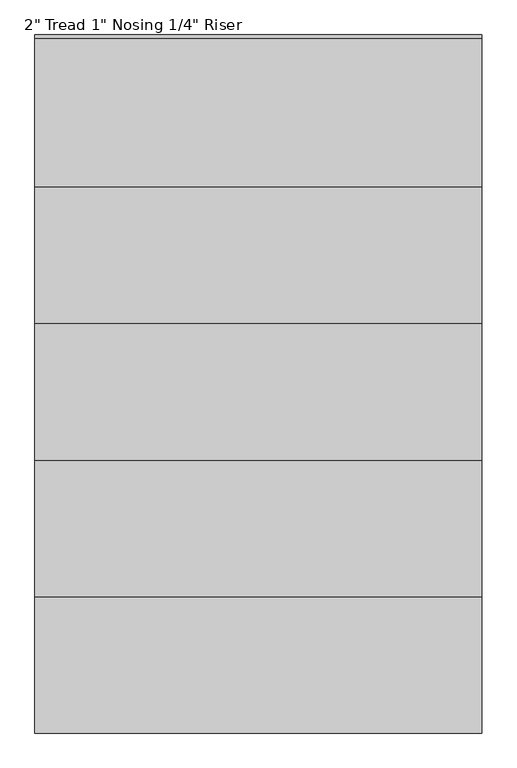
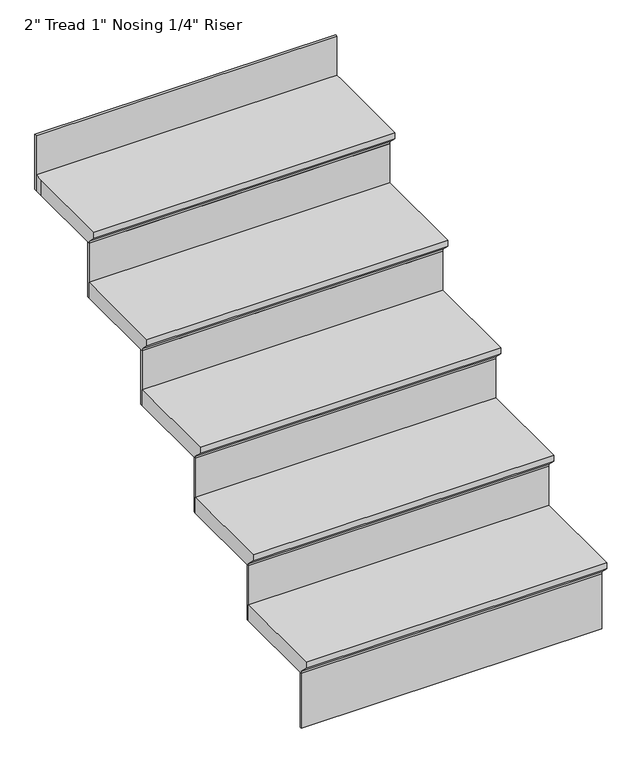
"""IFC4 building model written with IfcOpenShell, lengths in millimetres: stair flight geometry."""

from ifc_helpers import new_model, si_unit, origin, place, context, project, spatial, faceted_brep, source, transform, mapped, element, save


def stair_flight_150202ba(model_context):
    return source(origin(), model_context, "Body", "Brep", [
        faceted_brep([(9871.2423568, -9537.7746824, 1216.1921053), (9871.2423568, -9537.7746824, 1235.2421053), (8956.8423568, -9537.7746824, 1235.2421053), (8956.8423568, -9537.7746824, 1216.1921053), (9871.2423568, -9512.3746824, 1190.7921053), (8956.8423568, -9512.3746824, 1190.7921053), (9871.2423568, -9232.9746824, 1235.2421053), (8956.8423568, -9232.9746824, 1235.2421053), (8956.8423568, -9512.3746824, 1184.4421053), (8956.8423568, -9232.9746824, 1184.4421053), (9871.2423568, -9232.9746824, 1184.4421053), (9871.2423568, -9512.3746824, 1184.4421053)], [[[0, 1, 2, 3]], [[4, 0, 3, 5]], [[2, 1, 6, 7]], [[8, 9, 10, 11]], [[2, 7, 9, 8, 5, 3]], [[8, 11, 4, 5]], [[6, 1, 0, 4, 11, 10]], [[7, 6, 10, 9]]]),
        faceted_brep([(9871.2423568, -9512.3746824, 1184.4421053), (9871.2423568, -9512.3746824, 1007.9789474), (9871.2423568, -9506.0246824, 1007.9789474), (9871.2423568, -9506.0246824, 1184.4421053), (8956.8423568, -9512.3746824, 1184.4421053), (8956.8423568, -9506.0246824, 1184.4421053), (8956.8423568, -9506.0246824, 1007.9789474), (8956.8423568, -9512.3746824, 1007.9789474)], [[[0, 1, 2, 3]], [[4, 5, 6, 7]], [[1, 0, 4, 7]], [[2, 1, 7, 6]], [[3, 2, 6, 5]], [[0, 3, 5, 4]]]),
        faceted_brep([(9871.2423568, -9232.9746824, 1360.9052632), (9871.2423568, -9232.9746824, 1184.4421053), (9871.2423568, -9226.6246824, 1184.4421053), (9871.2423568, -9226.6246824, 1360.9052632), (8956.8423568, -9232.9746824, 1360.9052632), (8956.8423568, -9226.6246824, 1360.9052632), (8956.8423568, -9226.6246824, 1184.4421053), (8956.8423568, -9232.9746824, 1184.4421053)], [[[0, 1, 2, 3]], [[4, 5, 6, 7]], [[1, 0, 4, 7]], [[2, 1, 7, 6]], [[3, 2, 6, 5]], [[0, 3, 5, 4]]]),
        faceted_brep([(8956.8423568, -9258.3746824, 1411.7052632), (9871.2423568, -9258.3746824, 1411.7052632), (9871.2423568, -8953.5746824, 1411.7052632), (8956.8423568, -8953.5746824, 1411.7052632), (8956.8423568, -9232.9746824, 1360.9052632), (8956.8423568, -8953.5746824, 1360.9052632), (9871.2423568, -8953.5746824, 1360.9052632), (9871.2423568, -9232.9746824, 1360.9052632), (8956.8423568, -9232.9746824, 1367.2552632), (8956.8423568, -9258.3746824, 1392.6552632), (9871.2423568, -9232.9746824, 1367.2552632), (9871.2423568, -9258.3746824, 1392.6552632)], [[[0, 1, 2, 3]], [[4, 5, 6, 7]], [[0, 3, 5, 4, 8, 9]], [[4, 7, 10, 8]], [[2, 1, 11, 10, 7, 6]], [[3, 2, 6, 5]], [[11, 1, 0, 9]], [[10, 11, 9, 8]]]),
        faceted_brep([(9871.2423568, -8953.5746824, 1537.3684211), (9871.2423568, -8953.5746824, 1360.9052632), (9871.2423568, -8947.2246824, 1360.9052632), (9871.2423568, -8947.2246824, 1537.3684211), (8956.8423568, -8953.5746824, 1537.3684211), (8956.8423568, -8947.2246824, 1537.3684211), (8956.8423568, -8947.2246824, 1360.9052632), (8956.8423568, -8953.5746824, 1360.9052632)], [[[0, 1, 2, 3]], [[4, 5, 6, 7]], [[1, 0, 4, 7]], [[2, 1, 7, 6]], [[3, 2, 6, 5]], [[0, 3, 5, 4]]]),
        faceted_brep([(8956.8423568, -8978.9746824, 1588.1684211), (9871.2423568, -8978.9746824, 1588.1684211), (9871.2423568, -8674.1746824, 1588.1684211), (8956.8423568, -8674.1746824, 1588.1684211), (8956.8423568, -8953.5746824, 1537.3684211), (8956.8423568, -8674.1746824, 1537.3684211), (9871.2423568, -8674.1746824, 1537.3684211), (9871.2423568, -8953.5746824, 1537.3684211), (8956.8423568, -8953.5746824, 1543.7184211), (8956.8423568, -8978.9746824, 1569.1184211), (9871.2423568, -8953.5746824, 1543.7184211), (9871.2423568, -8978.9746824, 1569.1184211)], [[[0, 1, 2, 3]], [[4, 5, 6, 7]], [[0, 3, 5, 4, 8, 9]], [[4, 7, 10, 8]], [[2, 1, 11, 10, 7, 6]], [[3, 2, 6, 5]], [[11, 1, 0, 9]], [[10, 11, 9, 8]]]),
        faceted_brep([(9871.2423568, -8674.1746824, 1713.8315789), (9871.2423568, -8674.1746824, 1537.3684211), (9871.2423568, -8667.8246824, 1537.3684211), (9871.2423568, -8667.8246824, 1713.8315789), (8956.8423568, -8674.1746824, 1713.8315789), (8956.8423568, -8667.8246824, 1713.8315789), (8956.8423568, -8667.8246824, 1537.3684211), (8956.8423568, -8674.1746824, 1537.3684211)], [[[0, 1, 2, 3]], [[4, 5, 6, 7]], [[1, 0, 4, 7]], [[2, 1, 7, 6]], [[3, 2, 6, 5]], [[0, 3, 5, 4]]]),
        faceted_brep([(8956.8423568, -8699.5746824, 1764.6315789), (9871.2423568, -8699.5746824, 1764.6315789), (9871.2423568, -8394.7746824, 1764.6315789), (8956.8423568, -8394.7746824, 1764.6315789), (8956.8423568, -8674.1746824, 1713.8315789), (8956.8423568, -8394.7746824, 1713.8315789), (9871.2423568, -8394.7746824, 1713.8315789), (9871.2423568, -8674.1746824, 1713.8315789), (8956.8423568, -8674.1746824, 1720.1815789), (8956.8423568, -8699.5746824, 1745.5815789), (9871.2423568, -8674.1746824, 1720.1815789), (9871.2423568, -8699.5746824, 1745.5815789)], [[[0, 1, 2, 3]], [[4, 5, 6, 7]], [[0, 3, 5, 4, 8, 9]], [[4, 7, 10, 8]], [[2, 1, 11, 10, 7, 6]], [[3, 2, 6, 5]], [[11, 1, 0, 9]], [[10, 11, 9, 8]]]),
        faceted_brep([(9871.2423568, -8115.3746824, 2066.7578947), (9871.2423568, -8115.3746824, 1890.2947368), (9871.2423568, -8109.0246824, 1890.2947368), (9871.2423568, -8109.0246824, 2066.7578947), (8956.8423568, -8115.3746824, 2066.7578947), (8956.8423568, -8109.0246824, 2066.7578947), (8956.8423568, -8109.0246824, 1890.2947368), (8956.8423568, -8115.3746824, 1890.2947368)], [[[0, 1, 2, 3]], [[4, 5, 6, 7]], [[1, 0, 4, 7]], [[2, 1, 7, 6]], [[3, 2, 6, 5]], [[0, 3, 5, 4]]]),
        faceted_brep([(9871.2423568, -8394.7746824, 1890.2947368), (9871.2423568, -8394.7746824, 1713.8315789), (9871.2423568, -8388.4246824, 1713.8315789), (9871.2423568, -8388.4246824, 1890.2947368), (8956.8423568, -8394.7746824, 1890.2947368), (8956.8423568, -8388.4246824, 1890.2947368), (8956.8423568, -8388.4246824, 1713.8315789), (8956.8423568, -8394.7746824, 1713.8315789)], [[[0, 1, 2, 3]], [[4, 5, 6, 7]], [[1, 0, 4, 7]], [[2, 1, 7, 6]], [[3, 2, 6, 5]], [[0, 3, 5, 4]]]),
        faceted_brep([(8956.8423568, -8115.3746824, 1941.0947368), (8956.8423568, -8140.7746824, 1941.0947368), (8956.8423568, -8420.1746824, 1941.0947368), (9871.2423568, -8420.1746824, 1941.0947368), (9871.2423568, -8140.7746824, 1941.0947368), (9871.2423568, -8115.3746824, 1941.0947368), (8956.8423568, -8140.7746824, 1890.2947368), (8956.8423568, -8115.3746824, 1890.2947368), (9871.2423568, -8115.3746824, 1890.2947368), (9871.2423568, -8140.7746824, 1890.2947368), (9871.2423568, -8394.7746824, 1890.2947368), (8956.8423568, -8394.7746824, 1890.2947368), (8956.8423568, -8394.7746824, 1896.6447368), (8956.8423568, -8420.1746824, 1922.0447368), (9871.2423568, -8394.7746824, 1896.6447368), (9871.2423568, -8420.1746824, 1922.0447368)], [[[0, 1, 2, 3, 4, 5]], [[6, 7, 8, 9, 10, 11]], [[1, 0, 7, 6]], [[2, 1, 6, 11, 12, 13]], [[11, 10, 14, 12]], [[4, 3, 15, 14, 10, 9]], [[5, 4, 9, 8]], [[0, 5, 8, 7]], [[15, 3, 2, 13]], [[14, 15, 13, 12]]]),
    ])


if __name__ == "__main__":
    model = new_model("IFC4")
    model_context = context("Model", 3, world=origin())
    ifc_project = project(units=[si_unit("LENGTHUNIT", "METRE", prefix="MILLI")], contexts=[model_context])
    site = spatial("IfcSite", under=ifc_project)
    building = spatial("IfcBuilding", under=site)
    placement = place(None, origin())
    stair_flight_shape = stair_flight_150202ba(model_context)
    element("IfcStairFlight", 1, ObjectType="2\" Tread 1\" Nosing 1/4\" Riser", at=placement, inside=building, context=model_context, shape_type="MappedRepresentation", body=[
        mapped(stair_flight_shape, transform((0.0, 0.0, 0.0), x_axis=(1.0, 0.0, 0.0), y_axis=(0.0, 1.0, 0.0), z_axis=(0.0, 0.0, 1.0))),
    ])
    save(model, "model.ifc")

# Revit data of these elements
# Element 1 (IfcStairFlight, "2\" Tread 1\" Nosing 1/4\" Riser")
#   Materials on its faces: "MARBLE STAIRS 6\""
# Materials
#   "MARBLE STAIRS 6\"": class "Generic", colour RGB 120 120 120, transparency 0, Cost = 0
